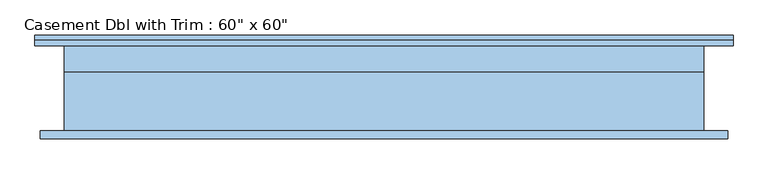
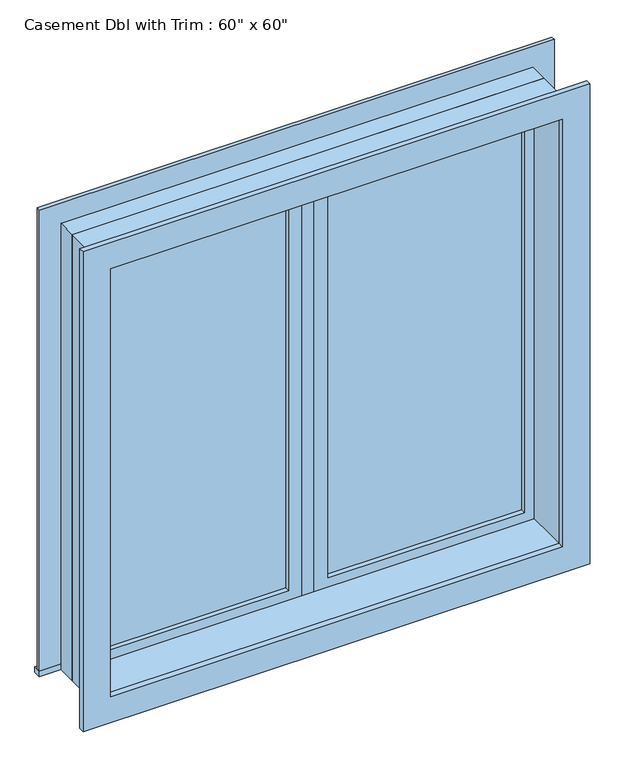
"""IFC4 building model written with IfcOpenShell, lengths in millimetres: window geometry."""

from ifc_helpers import new_model, si_unit, frame, origin, place, context, project, spatial, polyline, outline, extrude, source, transform, mapped, element, save


def window_514a67b1(model_context):
    return source(origin(), model_context, "Body", "SweptSolid", [
        extrude(outline(polyline([(63.5, 85.725), (698.5, 85.725), (698.5, 73.025), (63.5, 73.025), (63.5, 85.725)])), frame((0.0, 0.0, 977.9), z_axis=(0.0, 0.0, 1.0), x_axis=(1.0, 0.0, 0.0)), (0.0, 0.0, 1.0), 1397.0),
        extrude(outline(polyline([(2419.35, 19.05), (933.45, 19.05), (933.45, 742.95), (2419.35, 742.95), (2419.35, 19.05)]), holes=[polyline([(2374.9, 63.5), (2374.9, 698.5), (977.9, 698.5), (977.9, 63.5), (2374.9, 63.5)])]), frame((0.0, 57.15, 0.0), z_axis=(0.0, 1.0, 0.0), x_axis=(0.0, 0.0, 1.0)), (0.0, 0.0, 1.0), 44.45),
        extrude(outline(polyline([(19.05, 57.15), (-19.05, 57.15), (-19.05, 120.65), (19.05, 120.65), (19.05, 57.15)])), frame((0.0, 0.0, 933.45), z_axis=(0.0, 0.0, 1.0), x_axis=(1.0, 0.0, 0.0)), (0.0, 0.0, 1.0), 1485.9),
        extrude(outline(polyline([(-831.85, 146.05), (831.85, 146.05), (831.85, 120.65), (-831.85, 120.65), (-831.85, 146.05)])), frame((0.0, 0.0, 914.4), z_axis=(0.0, 0.0, 1.0), x_axis=(1.0, 0.0, 0.0)), (0.0, 0.0, 1.0), 19.05),
        extrude(outline(polyline([(2419.35, -742.95), (2419.35, 742.95), (933.45, 742.95), (933.45, 831.85), (2508.25, 831.85), (2508.25, -831.85), (933.45, -831.85), (933.45, -742.95), (2419.35, -742.95)])), frame((0.0, 120.65, 0.0), z_axis=(0.0, 1.0, 0.0), x_axis=(0.0, 0.0, 1.0)), (0.0, 0.0, 1.0), 12.7),
        extrude(outline(polyline([(2495.55, 819.15), (2495.55, -819.15), (857.25, -819.15), (857.25, 819.15), (2495.55, 819.15)]), holes=[polyline([(2406.65, 730.25), (946.15, 730.25), (946.15, -730.25), (2406.65, -730.25), (2406.65, 730.25)])]), frame((0.0, -101.6, 0.0), z_axis=(0.0, 1.0, 0.0), x_axis=(0.0, 0.0, 1.0)), (0.0, 0.0, 1.0), 19.05),
        extrude(outline(polyline([(-63.5, 73.025), (-698.5, 73.025), (-698.5, 85.725), (-63.5, 85.725), (-63.5, 73.025)])), frame((0.0, 0.0, 977.9), z_axis=(0.0, 0.0, 1.0), x_axis=(1.0, 0.0, 0.0)), (0.0, 0.0, 1.0), 1397.0),
        extrude(outline(polyline([(2419.35, -742.95), (933.45, -742.95), (933.45, -19.05), (2419.35, -19.05), (2419.35, -742.95)]), holes=[polyline([(2374.9, -698.5), (2374.9, -63.5), (977.9, -63.5), (977.9, -698.5), (2374.9, -698.5)])]), frame((0.0, 57.15, 0.0), z_axis=(0.0, 1.0, 0.0), x_axis=(0.0, 0.0, 1.0)), (0.0, 0.0, 1.0), 44.45),
        extrude(outline(polyline([(2438.4, -762.0), (914.4, -762.0), (914.4, 762.0), (2438.4, 762.0), (2438.4, -762.0)]), holes=[polyline([(2406.65, -730.25), (2406.65, 730.25), (946.15, 730.25), (946.15, -730.25), (2406.65, -730.25)])]), frame((0.0, -82.55, 0.0), z_axis=(0.0, 1.0, 0.0), x_axis=(0.0, 0.0, 1.0)), (0.0, 0.0, 1.0), 139.7),
        extrude(outline(polyline([(2438.4, 762.0), (2438.4, -762.0), (914.4, -762.0), (914.4, 762.0), (2438.4, 762.0)]), holes=[polyline([(2419.35, 742.95), (933.45, 742.95), (933.45, -742.95), (2419.35, -742.95), (2419.35, 742.95)])]), frame((0.0, 57.15, 0.0), z_axis=(0.0, 1.0, 0.0), x_axis=(0.0, 0.0, 1.0)), (0.0, 0.0, 1.0), 63.5),
    ])


if __name__ == "__main__":
    model = new_model("IFC4")
    model_context = context("Model", 3, world=origin())
    ifc_project = project(units=[si_unit("LENGTHUNIT", "METRE", prefix="MILLI")], contexts=[model_context])
    site = spatial("IfcSite", under=ifc_project)
    building = spatial("IfcBuilding", under=site)
    placement = place(None, origin())
    window_shape = window_514a67b1(model_context)
    element("IfcWindow", 1, ObjectType="Casement Dbl with Trim : 60\" x 60\"", at=placement, inside=building, context=model_context, shape_type="MappedRepresentation", body=[
        mapped(window_shape, transform((0.0, 0.0, 0.0), x_axis=(1.0, 0.0, 0.0), y_axis=(0.0, 1.0, 0.0), z_axis=(0.0, 0.0, 1.0))),
    ])
    save(model, "model.ifc")

# Revit data of these elements
# Type "Casement Dbl with Trim : 60\" x 60\""
#   Type Mark = "10"
#   Construction Type Id = "GSP4R"
#   Assembly Code = "B2020100"
#   Analytic Construction = "1/8 in Pilkington single glazing"
#   Visual Light Transmittance = 0.9
#   Thermal Resistance (R) = 1.53941 (h·ft²·°F)/BTU
#   Solar Heat Gain Coefficient = 0.78
#   Heat Transfer Coefficient (U) = 0.6496 BTU/(h·ft²·°F)
#   Height = 5' - 0"
#   Default Sill Height = 3' - 0"
#   Trim Projection - Ext. = 0' - 0 1/2"
#   Trim Projection - Int. = 0' - 0 3/4"
#   Trim Width - Exterior = 0' - 3 1/2"
#   Trim Width - Interior = 0' - 3 1/2"
#   Width = 5' - 0"
#   Window Inset = 0' - 0 3/4"
#   Define Thermal Properties by = 1
#   Glass Pane Material = Glass
#   Sash Material = Sash
#   Trim Exterior Material = Trim
#   Trim Interior Material = Roofing, EPDM Membrane
#   Wall Closure = (empty or 0)
# Element 1 (IfcWindow, "Casement Dbl with Trim : 60\" x 60\"")
#   Materials on its faces: "Sash", "Trim", "Glass", "Roofing, EPDM Membrane"
# Materials
#   "Glass": class "Glass", colour RGB 0 128 192, transparency 0.75, Description = "Soda Lime Glass", Cost = 0
#   "Sash": class "Wood", colour RGB 224 178 126, transparency 0
#   "Trim": class "Wood", colour RGB 224 178 126, transparency 0
#   "Roofing, EPDM Membrane": class "Generic", colour RGB 127 127 127, transparency 0, Description = "EPDM roof membrane", Cost = 0
